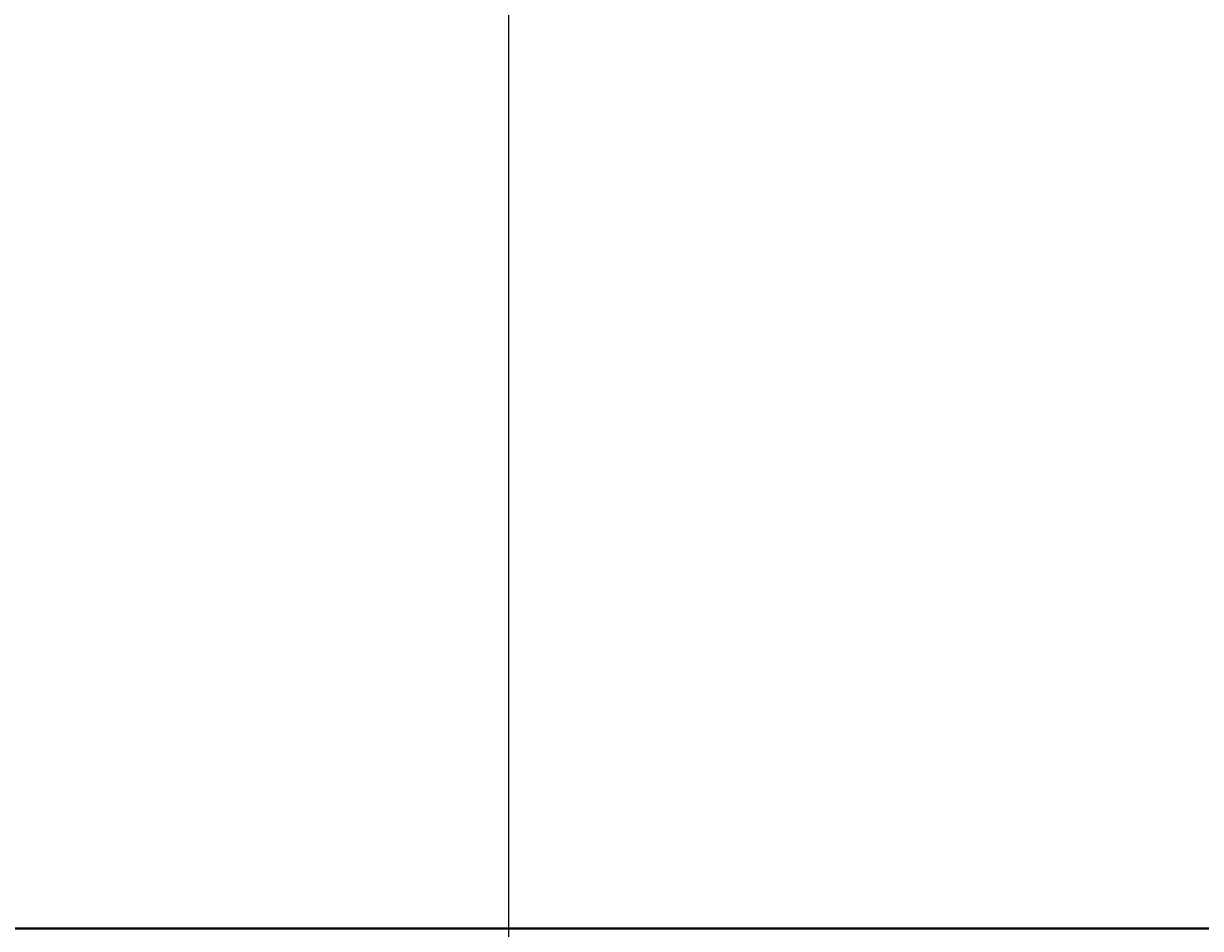
# Model space of a CAD drawing. Units: inches. Extents: x -301 to 715, y -607 to 364.
# Tile 61 of 141: x -144 to -93, y -215 to -176. Entities that reach past the tile are written whole.
import ezdxf

# ---------------------------------------------------------------- set-up
doc = ezdxf.new("R2010")
doc.units = ezdxf.units.IN
doc.header["$MEASUREMENT"] = 0
doc.layers.add('A-ANNO-DIMS', color=2, linetype='Continuous', lineweight=18)
doc.layers.add('A-WALL', color=3, linetype='Continuous', lineweight=40)
doc.styles.get("Standard").update_dxf_attribs({"font": 'arial.ttf'})
doc.dimstyles.get("Standard").update_dxf_attribs({"dimtxt": 0.18, "dimasz": 0.18, "dimexe": 0.18, "dimexo": 0.0625, "dimgap": 0.09, "dimtad": 0, "dimtih": 1, "dimtoh": 1, "dimdec": 1, "dimzin": 0, "dimdsep": 46, "dimlunit": 4, "dimtxsty": 'Standard', "dimcen": 0.09, "dimclrd": 3, "dimclre": 4, "dimclrt": 6, "dimadec": 0, "dimazin": 0, "dimtfac": 1, "dimtdec": 1, "dimtofl": 0, "dimtmove": 0, "dimatfit": 3, "dimfxl": 1, "dimtfill": 2, "dimtfillclr": 51, "dimtolj": 1, "dimtzin": 0, "dimarcsym": 0})

# ---------------------------------------------------------------- blocks, each defined once
blk = doc.blocks.new('*D151')
at = {"layer": 'A-ANNO-DIMS', "color": 4, "lineweight": -2, "transparency": 16777216}
for p, q in [((-204.603, -223.755), (-204.603, 359.612)), ((-45.603, -214.755), (-45.603, 359.612))]:
    blk.add_line(p, q, dxfattribs=at)
at = {"layer": 'A-ANNO-DIMS', "color": 3, "lineweight": -2, "transparency": 16777216}
for p, q in [((-204.423, 359.432), (-125.494, 359.432)), ((-45.783, 359.432), (-124.713, 359.432))]:
    blk.add_line(p, q, dxfattribs=at)
at = {"layer": 'A-ANNO-DIMS', "color": 3, "transparency": 16777216}
for points in [[(-204.423, 359.462), (-204.423, 359.402), (-204.603, 359.432)], [(-45.783, 359.462), (-45.783, 359.402), (-45.603, 359.432)]]:
    blk.add_solid(points, dxfattribs=at)
at = {"layer": 'Defpoints', "color": 0, "transparency": 16777216}
for p in [(-45.603, 359.432), (-45.603, -214.818), (-204.603, -223.818)]:
    blk.add_point(p, dxfattribs=at)
at = {"layer": 'A-ANNO-DIMS', "color": 6, "transparency": 16777216, "insert": (-125.103, 359.432), "char_height": 0.18, "attachment_point": 5, "bg_fill": 1, "box_fill_scale": 1.25, "bg_fill_color": 51, "bg_fill_transparency": 0}
blk.add_mtext('\\A1;13\'-3"', dxfattribs=at)
blk = doc.blocks.new('*D158')
at = {"layer": 'A-ANNO-DIMS', "color": 4, "lineweight": -2, "transparency": 16777216}
for p, q in [((-122.603, 221.62), (-122.603, -296.865)), ((-50.603, 221.62), (-50.603, -296.865))]:
    blk.add_line(p, q, dxfattribs=at)
at = {"layer": 'A-ANNO-DIMS', "color": 3, "lineweight": -2, "transparency": 16777216}
for p, q in [((-122.423, -296.685), (-86.933, -296.685)), ((-50.783, -296.685), (-86.274, -296.685))]:
    blk.add_line(p, q, dxfattribs=at)
at = {"layer": 'A-ANNO-DIMS', "color": 3, "transparency": 16777216}
for points in [[(-122.423, -296.655), (-122.423, -296.715), (-122.603, -296.685)], [(-50.783, -296.655), (-50.783, -296.715), (-50.603, -296.685)]]:
    blk.add_solid(points, dxfattribs=at)
at = {"layer": 'Defpoints', "color": 0, "transparency": 16777216}
for p in [(-122.603, 221.682), (-50.603, 221.682), (-50.603, -296.685)]:
    blk.add_point(p, dxfattribs=at)
at = {"layer": 'A-ANNO-DIMS', "color": 6, "transparency": 16777216, "insert": (-86.603, -296.685), "char_height": 0.18, "attachment_point": 5, "bg_fill": 1, "box_fill_scale": 1.25, "bg_fill_color": 51, "bg_fill_transparency": 0}
blk.add_mtext('\\A1;6\'-0"', dxfattribs=at)

msp = doc.modelspace()

# ---------------------------------------------------------------- linework, layer by layer
at = {"layer": 'A-WALL'}
msp.add_line((-195.603, -214.818), (-45.603, -214.818), dxfattribs=at)

# ---------------------------------------------------------------- dimensions: what is measured, and where the dimension line sits
at = {"layer": 'A-ANNO-DIMS'}
for base, p1, p2, picture, middle in [((-45.603, 359.432), (-204.603, -223.818), (-45.603, -214.818), '*D151', (-125.103, 359.432)), ((-50.603, -296.685), (-122.603, 221.682), (-50.603, 221.682), '*D158', (-86.603, -296.685))]:
    dim = msp.add_linear_dim(base=base, p1=p1, p2=p2, dimstyle='Standard', override={"dimdec": 1, "dimlfac": 1, "dimrnd": 0, "dimzin": 1, "dimdsep": 46, "dimlunit": 4, "dimfrac": 2}, dxfattribs=at)
    dim.commit()
    dim.dimension.update_dxf_attribs({"geometry": picture, "text_midpoint": middle})

doc.saveas('drawing.dxf')
